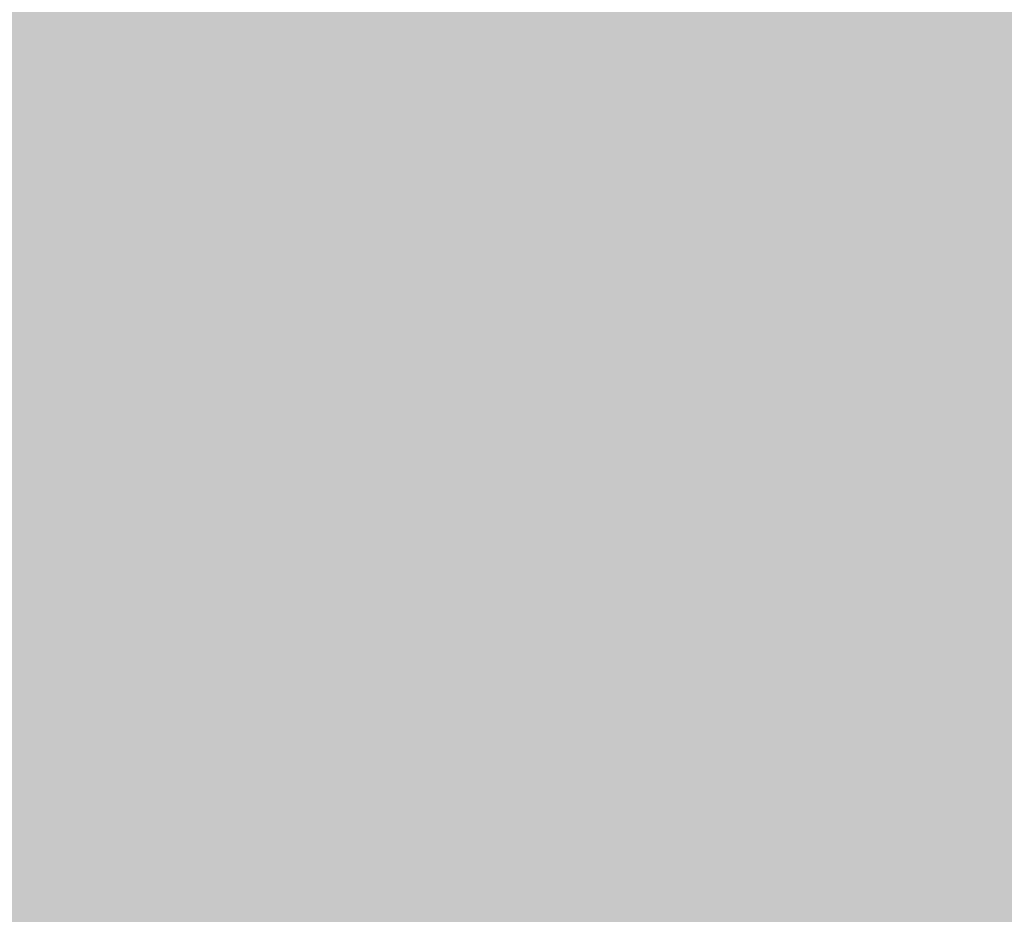
# Model space of a CAD drawing. Units: inches. Extents: x 2083 to 3317, y 1141 to 2115.
# Tile 42 of 256: x 2236.512 to 2237.1059, y 1477.1165 to 1477.6562. Entities that reach past the tile are written whole.
import ezdxf

# ---------------------------------------------------------------- set-up
doc = ezdxf.new("R2010")
doc.units = ezdxf.units.IN
doc.layers.add('A-ANNO-DIMS', color=2, linetype='Continuous', lineweight=18)
doc.layers.add('A-WALL-PATT', color=251, linetype='Continuous', lineweight=13, true_color=0x636466)
doc.styles.get("Standard").update_dxf_attribs({"font": 'arial.ttf'})
doc.dimstyles.new('ISO-25', dxfattribs={"dimtxt": 12, "dimasz": 12, "dimexe": 1.25, "dimexo": 0.625, "dimtad": 1, "dimlunit": 3, "dimtxsty": 'Standard', "dimcen": 2.5, "dimadec": 0, "dimazin": 0, "dimtfac": 1, "dimtmove": 0, "dimatfit": 3, "dimfxl": 1, "dimarcsym": 0})

# ---------------------------------------------------------------- blocks, each defined once
blk = doc.blocks.new('*D30')
at = {"layer": 'A-ANNO-DIMS', "color": 0, "lineweight": -2, "transparency": 16777216}
for p, q in [((2240.01786, 1445.27381), (2240.01786, 1448.04553)), ((2254.32933, 1445.27381), (2254.32933, 1448.04553)), ((2228.01786, 1446.79553), (2216.01786, 1446.79553)), ((2240.01786, 1446.79553), (2254.32933, 1446.79553)), ((2266.32933, 1446.79553), (2413.76487, 1446.79553))]:
    blk.add_line(p, q, dxfattribs=at)
at = {"layer": 'A-ANNO-DIMS', "color": 0, "transparency": 16777216}
for points in [[(2228.01786, 1448.79553), (2228.01786, 1444.79553), (2240.01786, 1446.79553)], [(2266.32933, 1448.79553), (2266.32933, 1444.79553), (2254.32933, 1446.79553)]]:
    blk.add_solid(points, dxfattribs=at)
at = {"layer": 'Defpoints', "color": 0, "transparency": 16777216}
for p in [(2254.32933, 1446.79553), (2240.01786, 1444.64881), (2254.32933, 1444.64881)]:
    blk.add_point(p, dxfattribs=at)
at = {"layer": 'A-ANNO-DIMS', "color": 0, "transparency": 16777216, "insert": (2346.0471, 1453.62517), "char_height": 12, "attachment_point": 5}
blk.add_mtext('WC 1\'-2 1/2" TYP.', dxfattribs=at)
blk = doc.blocks.new('*D31')
at = {"layer": 'A-ANNO-DIMS', "color": 0, "lineweight": -2, "transparency": 16777216}
for p, q in [((2237.87114, 1456.64881), (2237.87114, 1541.91518)), ((2239.39286, 1444.64881), (2236.62114, 1444.64881)), ((2237.87114, 1431.54754), (2237.87114, 1444.64881)), ((2239.39286, 1431.54754), (2236.62114, 1431.54754)), ((2237.87114, 1419.54754), (2237.87114, 1407.54754))]:
    blk.add_line(p, q, dxfattribs=at)
at = {"layer": 'A-ANNO-DIMS', "color": 0, "transparency": 16777216}
for points in [[(2235.87114, 1456.64881), (2239.87114, 1456.64881), (2237.87114, 1444.64881)], [(2235.87114, 1419.54754), (2239.87114, 1419.54754), (2237.87114, 1431.54754)]]:
    blk.add_solid(points, dxfattribs=at)
at = {"layer": 'Defpoints', "color": 0, "transparency": 16777216}
for p in [(2237.87114, 1444.64881), (2240.01786, 1444.64881), (2240.01786, 1431.54754)]:
    blk.add_point(p, dxfattribs=at)
at = {"layer": 'A-ANNO-DIMS', "color": 0, "transparency": 16777216, "insert": (2231.21749, 1505.28199), "char_height": 12, "attachment_point": 5, "rotation": 90}
blk.add_mtext('1\'-1" TYP.', dxfattribs=at)

msp = doc.modelspace()

# ---------------------------------------------------------------- hatches: boundary and pattern name
at = {"layer": 'A-WALL-PATT'}
h = msp.add_hatch(color=256, dxfattribs=at)
h.dxf.hatch_style = 1
h.paths.add_polyline_path([(3126.95978, 2020.76136), (2748.95978, 2020.76136), (2604.95978, 2020.76136), (2226.95978, 2020.76136), (2226.95978, 1702.76136), (2466.95978, 1702.76136), (2466.95978, 1582.76136), (2418.95978, 1582.76136), (2418.95978, 1477.76136), (2226.95978, 1477.76136), (2226.95978, 1263.26136), (2544.95978, 1263.26136), (2544.95978, 1411.76136), (2604.95978, 1411.76136), (2685.95978, 1411.76136), (2685.95978, 1420.76136), (2604.95978, 1420.76136), (2604.95978, 1573.76136), (2604.95978, 1702.76136), (2604.95978, 2011.76136), (2748.95978, 2011.76136), (2748.95978, 1702.76136), (2862.95978, 1702.76136), (2862.95978, 1621.76136), (2871.95978, 1621.76136), (2871.95978, 1702.76136), (2883.95978, 1702.76136), (2883.95978, 1706.93946, -0.026459), (2883.95978, 1711.76136), (2757.95978, 1711.76136), (2757.95978, 1807.76136), (2787.95978, 1807.76136), (2787.95978, 1812.26136), (2757.95978, 1812.26136), (2757.95978, 2011.76136), (2877.95978, 2011.76136), (2877.95978, 1812.26136), (2847.95978, 1812.26136), (2847.95978, 1807.76136), (2889.83574, 1807.76136), (2889.83574, 1812.26136), (2882.45978, 1812.26136), (2882.45978, 2011.76136), (3117.95978, 2011.76136), (3117.95978, 1812.26136), (2937.83574, 1812.26136), (2937.83574, 1807.76136), (2995.70978, 1807.76136), (2995.70978, 1796.11767), (3000.20978, 1796.11767), (3000.20978, 1807.76136), (3117.95978, 1807.76136), (3117.95978, 1711.76136), (3000.20978, 1711.76136), (3000.20978, 1760.11767), (2998.5727, 1760.11767, -0.020711), (2995.70978, 1760.11767), (2995.70978, 1711.76136), (2931.95978, 1711.76136), (2931.95978, 1702.76136), (3126.95978, 1702.76136)])
h.paths.add_polyline_path([(2471.45978, 2011.76136), (2471.45978, 1810.01136), (2462.71694, 1810.01136), (2462.71694, 1805.51136), (2505.95978, 1805.51136), (2505.95978, 1810.01136), (2475.95978, 1810.01136), (2475.95978, 2011.76136), (2595.95978, 2011.76136), (2595.95978, 1810.01136), (2565.95978, 1810.01136), (2565.95978, 1805.51136), (2595.95978, 1805.51136), (2595.95978, 1711.76136), (2235.95978, 1711.76136), (2235.95978, 1805.51136), (2353.70978, 1805.51136), (2353.70978, 1796.05416), (2358.20978, 1796.05416), (2358.20978, 1805.51136), (2414.71694, 1805.51136), (2414.71694, 1810.01136), (2235.95978, 1810.01136), (2235.95978, 2011.76136)], flags=16)
h.paths.add_polyline_path([(2270.20473, 1994.61001), (2270.20473, 1970.61001), (2246.20473, 1970.61001), (2246.20473, 1994.61001)], flags=0)
edge = h.paths.add_edge_path(flags=0)
edge.add_ellipse((2332.02739, 1899.79818), major_axis=(-3.04299, 3.04299), ratio=0.1682525, start_angle=-161.33217, end_angle=-156.30711, ccw=False)
edge.add_ellipse((2333.08204, 1898.74353), major_axis=(-1.05465, 1.05465), ratio=0.4535321, start_angle=-123.37102, end_angle=-94.15911)
edge = h.paths.add_edge_path(flags=0)
edge.add_ellipse((2332.02739, 1968.87629), major_axis=(3.04299, 3.04299), ratio=0.1682525, start_angle=18.66783, end_angle=23.69289)
edge.add_spline(control_points=[(2332.9256, 1970.6911), (2332.22677, 1970.3361), (2330.89371, 1969.65891), (2328.41308, 1970.93214), (2327.20393, 1967.74871), (2324.7096, 1969.95559), (2322.53282, 1967.01235), (2320.01285, 1971.29581), (2317.68031, 1968.15784), (2316.04053, 1967.10205), (2315.4269, 1966.8096)], knot_values=[0, 0, 0, 0, 2.267059, 4.324559, 6.685584, 8.878641, 11.121502, 14.300359, 17.755284, 19.732645, 19.732645, 19.732645, 19.732645], degree=3, periodic=0)
edge.add_ellipse((2332.02739, 1968.87629), major_axis=(3.04299, 3.04299), ratio=0.1682525, start_angle=18.66783, end_angle=23.69289, ccw=False)
edge.add_ellipse((2333.08204, 1969.93094), major_axis=(1.05465, 1.05465), ratio=0.4535321, start_angle=56.62898, end_angle=85.84089, ccw=False)
edge = h.paths.add_edge_path(flags=0)
edge.add_spline(control_points=[(2296.42829, 1967.98791), (2293.6278, 1965.33631), (2287.70362, 1959.72709), (2299.74386, 1949.9957), (2294.53259, 1935.66853), (2290.57323, 1920.60351), (2293.39412, 1909.97369), (2296.18541, 1904.96654)], knot_values=[0.099185, 0.099185, 0.099185, 0.099185, 0.345301, 0.619822, 0.982653, 1.386093, 1.810555, 1.810555, 1.810555, 1.810555], degree=3, periodic=0)
edge.add_spline(control_points=[(2296.18541, 1904.96654), (2297.38358, 1902.6193), (2298.00097, 1901.94931), (2298.55297, 1901.46815)], knot_values=[0.006246, 0.006246, 0.006246, 0.006246, 0.055476, 0.055476, 0.055476, 0.055476], degree=3, periodic=0)
edge.add_spline(control_points=[(2298.55297, 1901.46815), (2297.25861, 1900.92322), (2295.22529, 1900.23213), (2293.06023, 1900.61421), (2292.10142, 1900.78841), (2292.08958, 1900.79057)], knot_values=[0.312835, 0.312835, 0.312835, 0.312835, 0.40178, 0.474987, 0.475903, 0.475903, 0.475903, 0.475903], degree=3, periodic=0)
edge.add_arc((2292.79365, 1904.66411), 3.93701, 215.4209, 259.69818, ccw=False)
edge.add_spline(control_points=[(2289.58531, 1902.3823), (2289.47665, 1902.53509), (2289.36848, 1902.68804), (2289.26086, 1902.84117)], knot_values=[0.102872, 0.102872, 0.102872, 0.102872, 0.116896, 0.116896, 0.116896, 0.116896], degree=3, periodic=0)
edge.add_spline(control_points=[(2289.26086, 1902.84117), (2288.6866, 1902.55019), (2287.64005, 1902.0199), (2285.88134, 1901.87395), (2283.85297, 1901.50435), (2281.71999, 1899.71054), (2278.46699, 1899.49294), (2276.15714, 1901.8832), (2272.25895, 1899.80407), (2267.77761, 1901.84318), (2262.24388, 1900.18403), (2257.41493, 1901.78206), (2254.31837, 1900.72612), (2253.17828, 1900.33734)], knot_values=[0, 0, 0, 0, 1.907977, 3.477176, 5.261074, 7.972851, 11.680248, 13.717921, 16.939592, 22.789562, 27.502503, 33.595215, 37.145618, 37.145618, 37.145618, 37.145618], degree=3, periodic=0)
edge.add_line((2253.17828, 1900.33734), (2250.24424, 1902.84117))
edge.add_line((2250.24424, 1902.84117), (2250.24424, 1965.8333))
edge.add_line((2250.24424, 1965.8333), (2253.17828, 1968.33712))
edge.add_spline(control_points=[(2253.17828, 1968.33712), (2254.31837, 1967.94835), (2257.41493, 1966.89241), (2262.24388, 1968.49043), (2267.77761, 1966.83128), (2271.52673, 1968.53722), (2273.87591, 1967.82829), (2274.2067, 1967.72764)], knot_values=[0, 0, 0, 0, 0.09018, 0.244935, 0.364644, 0.513233, 0.537855, 0.537855, 0.537855, 0.537855], degree=3, periodic=0)
edge.add_arc((2274.35289, 1963.79335), 3.93701, 72.05113, 92.12795, ccw=False)
edge.add_arc((2281.29693, 1985.23), 18.5963, 252.051134, 288.565722)
edge.add_arc((2292.31672, 1956.02888), 12.64608, 71.026788, 113.778218, ccw=False)
edge = h.paths.add_edge_path(flags=0)
edge.add_spline(control_points=[(2274.89941, 1951.85619), (2275.06616, 1951.61659), (2275.23269, 1951.37659), (2275.39799, 1951.13585)], knot_values=[1.409916, 1.409916, 1.409916, 1.409916, 1.43159, 1.43159, 1.43159, 1.43159], degree=3, periodic=0)
edge.add_spline(control_points=[(2275.39799, 1951.13585), (2275.79211, 1950.56189), (2276.17923, 1949.98377), (2276.54555, 1949.3971)], knot_values=[1.358238, 1.358238, 1.358238, 1.358238, 1.409916, 1.409916, 1.409916, 1.409916], degree=3, periodic=0)
edge.add_line((2276.54555, 1949.3971), (2277.43729, 1947.86218))
edge.add_spline(control_points=[(2277.43729, 1947.86218), (2276.30383, 1945.67311), (2274.6397, 1942.42688), (2274.63161, 1938.0939), (2272.79912, 1930.85155), (2274.35643, 1943.89705), (2275.94768, 1947.92336), (2276.54555, 1949.3971)], knot_values=[0.005632, 0.005632, 0.005632, 0.005632, 0.186014, 0.266002, 0.357087, 0.59639, 0.739732, 0.739732, 0.739732, 0.739732], degree=3, periodic=0)
edge.add_spline(control_points=[(2276.54555, 1949.3971), (2276.17923, 1949.98377), (2275.79211, 1950.56189), (2275.39799, 1951.13585)], knot_values=[1.358238, 1.358238, 1.358238, 1.358238, 1.409916, 1.409916, 1.409916, 1.409916], degree=3, periodic=0)
edge.add_spline(control_points=[(2275.39799, 1951.13585), (2274.9425, 1950.08045), (2274.20776, 1948.02527), (2273.9346, 1944.85148), (2272.46853, 1937.62749), (2273.46622, 1945.69647), (2274.70062, 1951.05947), (2274.89941, 1951.85619)], knot_values=[0.104364, 0.104364, 0.104364, 0.104364, 0.189636, 0.269624, 0.36071, 0.600013, 0.644622, 0.644622, 0.644622, 0.644622], degree=3, periodic=0)
h.paths.add_polyline_path([(2269.16751, 1963.12757, -0.357527), (2268.17063, 1960.97637, -0.092561), (2268.17063, 1939.43632, -0.357527), (2269.16751, 1937.28512, -0.357527), (2267.01631, 1938.282, -0.164785), (2254.68558, 1938.282, -0.357527), (2252.53438, 1937.28512, -0.357527), (2253.53126, 1939.43632, -0.092561), (2253.53126, 1960.97637, -0.357527), (2252.53438, 1963.12757, -0.357527), (2254.68558, 1962.13069, -0.164785), (2267.01631, 1962.13069, -0.357527)], flags=0)
h.paths.add_polyline_path([(2248.87407, 1967.8018), (2248.87407, 1957.02771), (2249.45778, 1957.02771), (2249.45778, 1911.64676), (2248.87407, 1911.64676), (2248.87407, 1900.87267), (2246.51186, 1900.87267, 0.197327), (2244.14966, 1902.45687), (2244.14966, 1966.21759, 0.197327), (2246.51186, 1967.8018)], flags=0)
h.paths.add_polyline_path([(2269.16751, 1931.38934, -0.357527), (2268.17063, 1929.23814, -0.092561), (2268.17063, 1907.6981, -0.357527), (2269.16751, 1905.54689, -0.357527), (2267.01631, 1906.54377, -0.164785), (2254.68558, 1906.54377, -0.357527), (2252.53438, 1905.54689, -0.357527), (2253.53126, 1907.6981, -0.092561), (2253.53126, 1929.23814, -0.357527), (2252.53438, 1931.38934, -0.357527), (2254.68558, 1930.39246, -0.164785), (2267.01631, 1930.39246, -0.357527)], flags=0)
edge = h.paths.add_edge_path(flags=0)
edge.add_spline(control_points=[(2276.19686, 1906.7237), (2276.16814, 1909.02893), (2276.11405, 1913.37185), (2270.59842, 1924.92498), (2273.90517, 1919.01278), (2275.92171, 1916.26206), (2275.47457, 1912.40215), (2277.25787, 1910.38062), (2276.69604, 1908.22504), (2276.64622, 1906.81302), (2276.61782, 1906.00841)], knot_values=[0, 0, 0, 0, 8.61026, 16.221274, 18.843057, 23.804898, 27.440828, 29.356102, 31.203478, 33.650687, 33.650687, 33.650687, 33.650687], degree=3, periodic=0)
edge.add_spline(control_points=[(2276.61782, 1906.00841), (2276.62331, 1905.62414), (2276.49774, 1904.62866), (2275.44178, 1903.85473), (2274.93731, 1903.08045), (2274.85908, 1902.84117)], knot_values=[0.156488, 0.156488, 0.156488, 0.156488, 0.184398, 0.231376, 0.250598, 0.250598, 0.250598, 0.250598], degree=3, periodic=0)
edge.add_line((2274.85908, 1902.84117), (2276.50598, 1902.84117))
edge.add_spline(control_points=[(2276.50598, 1902.84117), (2276.78831, 1903.08494), (2277.66507, 1904.1252), (2278.24954, 1904.34074), (2277.65387, 1908.52739), (2278.15567, 1906.22781), (2278.10046, 1905.28595), (2278.84667, 1904.06901), (2277.85679, 1903.41495), (2277.87419, 1902.99105), (2277.90356, 1902.84117)], knot_values=[0.059574, 0.059574, 0.059574, 0.059574, 0.080753, 0.103741, 0.16972, 0.176036, 0.207137, 0.240474, 0.262341, 0.27366, 0.27366, 0.27366, 0.27366], degree=3, periodic=0)
edge.add_line((2277.90356, 1902.84117), (2280.02983, 1902.84117))
edge.add_spline(control_points=[(2280.02983, 1902.84117), (2279.88822, 1903.0884), (2279.49926, 1903.98155), (2280.15228, 1905.93935), (2278.10362, 1909.65776), (2279.76239, 1907.18529), (2280.3279, 1904.87486), (2280.48511, 1903.48959), (2281.46327, 1903.24943), (2281.75834, 1902.9365), (2281.83404, 1902.84117)], knot_values=[0.013856, 0.013856, 0.013856, 0.013856, 0.034874, 0.088867, 0.107879, 0.126738, 0.158714, 0.193757, 0.217487, 0.226722, 0.226722, 0.226722, 0.226722], degree=3, periodic=0)
edge.add_spline(control_points=[(2281.83404, 1902.84117), (2281.78753, 1902.8267), (2281.64702, 1902.78299), (2281.39553, 1902.85949), (2281.08808, 1902.98524), (2280.72068, 1903.0609), (2280.33345, 1903.02573), (2280.12477, 1902.89888), (2280.02983, 1902.84117)], knot_values=[0, 0, 0, 0, 0.14413, 0.435517, 0.749276, 1.153046, 1.548371, 1.878348, 1.878348, 1.878348, 1.878348], degree=3, periodic=0)
edge.add_line((2280.02983, 1902.84117), (2277.90356, 1902.84117))
edge.add_spline(control_points=[(2277.90356, 1902.84117), (2277.89286, 1902.79586), (2277.8654, 1902.67964), (2277.60748, 1902.68748), (2277.27405, 1902.8007), (2276.83792, 1902.61977), (2276.58381, 1902.78926), (2276.50598, 1902.84117)], knot_values=[0, 0, 0, 0, 0.127189, 0.326199, 0.628009, 1.24357, 1.515331, 1.515331, 1.515331, 1.515331], degree=3, periodic=0)
edge.add_line((2276.50598, 1902.84117), (2274.85908, 1902.84117))
edge.add_spline(control_points=[(2274.85908, 1902.84117), (2274.81444, 1902.89859), (2274.72513, 1903.01345), (2274.49348, 1903.11897), (2274.24429, 1902.96054), (2273.93712, 1903.18494), (2273.61404, 1902.98314), (2273.40832, 1902.88304), (2273.32225, 1902.84117)], knot_values=[0, 0, 0, 0, 0.21843, 0.436957, 0.687977, 0.990379, 1.398396, 1.69185, 1.69185, 1.69185, 1.69185], degree=3, periodic=0)
edge.add_spline(control_points=[(2273.32225, 1902.84117), (2273.61674, 1903.44569), (2274.274, 1904.53825), (2276.02724, 1904.5737), (2276.20696, 1906.58364), (2276.19686, 1906.7237)], knot_values=[0.012227, 0.012227, 0.012227, 0.012227, 0.059472, 0.106218, 0.134458, 0.134458, 0.134458, 0.134458], degree=3, periodic=0)
h.paths.add_polyline_path([(2270.77605, 1897.78983), (2270.77605, 1873.78983), (2246.77605, 1873.78983), (2246.77605, 1897.78983)], flags=0)
h.paths.add_polyline_path([(2353.70978, 1760.00506), (2353.70978, 1760.05416), (2358.20978, 1760.05416, -0.033729)], flags=0)
h.paths.add_polyline_path([(2321.81912, 1737.52919), (2341.99533, 1737.52919, -0.414214), (2343.20327, 1736.32124), (2343.20327, 1721.0206, -0.414214), (2341.99533, 1719.81265), (2321.81912, 1719.81265, -0.414214), (2320.61117, 1721.0206), (2320.61117, 1736.32124, -0.414214)], flags=0)
h.paths.add_polyline_path([(2324.23501, 1736.32124), (2339.57944, 1736.32124, -0.414214), (2341.99533, 1733.90535), (2341.99533, 1725.44973, -0.414214), (2339.57944, 1723.03384), (2333.68059, 1723.03384), (2333.84532, 1722.04547, -0.870646), (2335.4254, 1721.82589, -0.767327), (2333.92269, 1721.42324), (2331.29102, 1721.42324, -0.767327), (2329.78832, 1721.82589, -0.870646), (2331.3684, 1722.04547), (2331.53313, 1723.03384), (2324.23501, 1723.03384, -0.414214), (2321.81912, 1725.44973), (2321.81912, 1733.90535, -0.414214)], flags=0)
h.paths.add_polyline_path([(2570.48379, 1928.61544), (2589.68379, 1928.61544), (2590.16883, 1928.61544), (2590.16883, 1904.9934), (2570.48379, 1904.9934)], flags=0)
h.paths.add_polyline_path([(2574.44732, 1927.26382, -1), (2572.82884, 1927.26382, -1)], flags=0)
h.paths.add_polyline_path([(2573.08987, 1926.94088), (2573.92503, 1927.77604), (2574.14774, 1927.55333), (2573.31258, 1926.71817)], flags=0)
h.paths.add_polyline_path([(2578.77906, 1919.72962, -1), (2571.59166, 1919.72962, -1)], flags=0)
h.paths.add_polyline_path([(2578.38536, 1919.72962, -1), (2571.98536, 1919.72962, -1)], flags=0)
h.paths.add_polyline_path([(2331.59576, 1729.47622, -1), (2333.61795, 1729.47622, -1)], flags=0)
h.paths.add_polyline_path([(2578.03423, 1927.26382, -1), (2576.41574, 1927.26382, -1)], flags=0)
h.paths.add_polyline_path([(2576.68885, 1927.53109), (2576.91156, 1927.7538), (2577.74673, 1926.91863), (2577.52402, 1926.69592)], flags=0)
h.paths.add_polyline_path([(2578.13906, 1909.85954, -1), (2572.23166, 1909.85954, -1)], flags=0)
h.paths.add_polyline_path([(2577.74536, 1909.85954, -1), (2572.62536, 1909.85954, -1)], flags=0)
h.paths.add_polyline_path([(2583.79772, 1927.26382, -1), (2582.17923, 1927.26382, -1)], flags=0)
h.paths.add_polyline_path([(2582.71865, 1927.7538), (2583.55381, 1926.91863), (2583.3311, 1926.69592), (2582.49594, 1927.53109)], flags=0)
h.paths.add_polyline_path([(2582.49594, 1927.53109), (2582.71865, 1927.7538), (2583.55381, 1926.91863), (2583.3311, 1926.69592)], flags=0)
h.paths.add_polyline_path([(2587.73906, 1920.52962, -1), (2581.83166, 1920.52962, -1)], flags=0)
h.paths.add_polyline_path([(2587.34536, 1920.52962, -1), (2582.22536, 1920.52962, -1)], flags=0)
h.paths.add_polyline_path([(2587.38462, 1927.26382, -1), (2585.76613, 1927.26382, -1)], flags=0)
h.paths.add_polyline_path([(2586.08199, 1926.98025), (2586.91716, 1927.81541), (2587.13987, 1927.5927), (2586.3047, 1926.75754)], flags=0)
h.paths.add_polyline_path([(2588.37906, 1910.65954, -1), (2581.19166, 1910.65954, -1)], flags=0)
h.paths.add_polyline_path([(2587.98536, 1910.65954, -1), (2581.58536, 1910.65954, -1)], flags=0)
h.paths.add_polyline_path([(2417.16773, 1729.4779), (2437.34394, 1729.4779, -0.414214), (2438.55188, 1728.26995), (2438.55188, 1712.96931, -0.414214), (2437.34394, 1711.76136), (2417.16773, 1711.76136, -0.414214), (2415.95978, 1712.96931), (2415.95978, 1728.26995, -0.414214)], flags=0)
h.paths.add_polyline_path([(2419.58362, 1728.26995), (2434.92805, 1728.26995, -0.414214), (2437.34394, 1725.85406), (2437.34394, 1717.39844, -0.414214), (2434.92805, 1714.98255), (2429.0292, 1714.98255), (2429.19393, 1713.99418, -0.870646), (2430.77401, 1713.7746, -0.767327), (2429.2713, 1713.37195), (2426.63963, 1713.37195, -0.767327), (2425.13693, 1713.7746, -0.870646), (2426.71701, 1713.99418), (2426.88174, 1714.98255), (2419.58362, 1714.98255, -0.414214), (2417.16773, 1717.39844), (2417.16773, 1725.85406, -0.414214)], flags=0)
h.paths.add_polyline_path([(2419.58362, 1728.26995), (2434.92805, 1728.26995, -0.414214), (2437.34394, 1725.85406), (2437.34394, 1717.39844, -0.414214), (2434.92805, 1714.98255), (2429.0292, 1714.98255), (2428.35812, 1719.00903), (2427.55282, 1719.00903), (2426.88174, 1714.98255), (2419.58362, 1714.98255, -0.414214), (2417.16773, 1717.39844), (2417.16773, 1725.85406, -0.414214)], flags=0)
h.paths.add_polyline_path([(2426.94437, 1721.42492, -1), (2428.96656, 1721.42492, -1)], flags=0)
h.paths.add_polyline_path([(2475.95978, 1702.76136), (2595.95978, 1702.76136), (2595.95978, 1582.76136), (2475.95978, 1582.76136)], flags=16)
h.paths.add_polyline_path([(2427.95978, 1573.76136), (2595.95978, 1573.76136), (2595.95978, 1468.76136), (2595.95978, 1420.76136), (2384.45978, 1420.76136), (2384.45978, 1468.76136), (2427.95978, 1468.76136)], flags=16)
h.paths.add_polyline_path([(2379.95978, 1468.76136), (2379.95978, 1420.76136), (2235.95978, 1420.76136), (2235.95978, 1468.76136)], flags=16)
h.paths.add_polyline_path([(2317.816, 1466.69577), (2337.9922, 1466.69577, -0.414214), (2339.20015, 1465.48782), (2339.20015, 1450.18718, -0.414214), (2337.9922, 1448.97923), (2317.816, 1448.97923, -0.414214), (2316.60805, 1450.18718), (2316.60805, 1465.48782, -0.414214)], flags=0)
h.paths.add_polyline_path([(2320.23189, 1465.48782), (2335.57631, 1465.48782, -0.414214), (2337.9922, 1463.07193), (2337.9922, 1454.61631, -0.414214), (2335.57631, 1452.20042), (2329.67747, 1452.20042), (2329.84219, 1451.21205, -0.870646), (2331.42228, 1450.99247, -0.767327), (2329.91957, 1450.58983), (2327.2879, 1450.58983, -0.767327), (2325.7852, 1450.99247, -0.870646), (2327.36528, 1451.21205), (2327.53001, 1452.20042), (2320.23189, 1452.20042, -0.414214), (2317.816, 1454.61631), (2317.816, 1463.07193, -0.414214)], flags=0)
h.paths.add_polyline_path([(2320.23189, 1465.48782), (2335.57631, 1465.48782, -0.414214), (2337.9922, 1463.07193), (2337.9922, 1454.61631, -0.414214), (2335.57631, 1452.20042), (2329.67747, 1452.20042), (2329.00638, 1456.22691), (2328.20109, 1456.22691), (2327.53001, 1452.20042), (2320.23189, 1452.20042, -0.414214), (2317.816, 1454.61631), (2317.816, 1463.07193, -0.414214)], flags=0)
h.paths.add_polyline_path([(2327.59264, 1458.6428, -1), (2329.61483, 1458.6428, -1)], flags=0)
h.paths.add_polyline_path([(2244.41174, 1433.34045), (2241.92094, 1433.34045, -0.414214), (2240.01786, 1435.24354), (2240.01786, 1440.95281, -0.414211), (2241.92093, 1442.8559), (2244.41174, 1442.8559, -1.976472)], flags=0)
h.paths.add_polyline_path([(2245.35689, 1434.39754, -0.414214), (2245.35689, 1441.79881, -2.144098)], flags=0)
h.paths.add_polyline_path([(2535.95978, 1416.26136), (2535.95978, 1272.26136), (2235.95978, 1272.26136), (2235.95978, 1416.26136)], flags=16)
h.paths.add_polyline_path([(2260.11956, 1384.29284), (2260.11956, 1362.03865), (2237.86537, 1362.03865), (2237.86537, 1384.29284)], flags=0)
edge = h.paths.add_edge_path(flags=0)
edge.add_line((2318.25185, 1362.0933), (2318.1458, 1362.00097))
edge.add_ellipse((2317.44512, 1360.43104), major_axis=(2.82164, 2.82164), ratio=0.1682525, start_angle=18.66783, end_angle=20.94813, ccw=False)
edge.add_ellipse((2318.42305, 1361.40897), major_axis=(0.97793, 0.97793), ratio=0.4535321, start_angle=56.62898, end_angle=70.2262, ccw=False)
edge = h.paths.add_edge_path(flags=0)
edge.add_line((2319.10737, 1295.57108), (2319.01504, 1295.67713))
edge.add_ellipse((2317.44512, 1296.37781), major_axis=(-2.82164, 2.82164), ratio=0.1682525, start_angle=-161.33217, end_angle=-159.05187, ccw=False)
edge.add_ellipse((2318.42305, 1295.39988), major_axis=(-0.97793, 0.97793), ratio=0.4535321, start_angle=-123.37102, end_angle=-109.7738)
edge = h.paths.add_edge_path(flags=0)
edge.add_spline(control_points=[(2284.21035, 1301.17022), (2284.58069, 1300.44472), (2284.89119, 1299.89202), (2285.15955, 1299.46102)], knot_values=[0.039066, 0.039066, 0.039066, 0.039066, 0.055476, 0.055476, 0.055476, 0.055476], degree=3, periodic=0)
edge.add_line((2285.15955, 1299.46102), (2284.21035, 1301.17022))
edge = h.paths.add_edge_path(flags=0)
edge.add_line((2280.41246, 1297.29801), (2283.36999, 1297.03612))
edge.add_line((2283.36999, 1297.03612), (2286.40569, 1297.92631))
edge.add_spline(control_points=[(2286.40569, 1297.92631), (2285.30549, 1297.46312), (2284.34478, 1297.12915), (2283.36999, 1297.03612)], knot_values=[0.394369, 0.394369, 0.394369, 0.394369, 0.475903, 0.475903, 0.475903, 0.475903], degree=3, periodic=0)
edge.add_spline(control_points=[(2283.36999, 1297.03612), (2283.28139, 1297.02767), (2282.31629, 1296.95734), (2281.3125, 1297.13448), (2280.42344, 1297.29602), (2280.41246, 1297.29801)], knot_values=[0.312835, 0.312835, 0.312835, 0.312835, 0.320246, 0.393453, 0.394369, 0.394369, 0.394369, 0.394369], degree=3, periodic=0)
edge = h.paths.add_edge_path(flags=0)
edge.add_line((2284.43556, 1359.60729), (2280.44629, 1355.32805))
edge.add_line((2280.44629, 1355.32805), (2279.57999, 1351.01775))
edge.add_line((2279.57999, 1351.01775), (2282.41297, 1346.58043))
edge.add_spline(control_points=[(2282.41297, 1346.58043), (2283.15333, 1345.58924), (2284.2529, 1344.0289), (2284.80104, 1342.38717), (2284.93516, 1341.80554)], knot_values=[1.240098, 1.240098, 1.240098, 1.240098, 1.332892, 1.382712, 1.382712, 1.382712, 1.382712], degree=3, periodic=0)
edge.add_spline(control_points=[(2284.93516, 1341.80554), (2285.31911, 1340.1406), (2285.23303, 1338.4092), (2284.90994, 1336.65412)], knot_values=[1.097484, 1.097484, 1.097484, 1.097484, 1.240098, 1.240098, 1.240098, 1.240098], degree=3, periodic=0)
edge.add_spline(control_points=[(2284.90994, 1336.65412), (2284.58685, 1334.89904), (2284.02675, 1333.12027), (2283.46264, 1331.36058)], knot_values=[0.95487, 0.95487, 0.95487, 0.95487, 1.097484, 1.097484, 1.097484, 1.097484], degree=3, periodic=0)
edge.add_line((2283.46264, 1331.36058), (2281.89038, 1326.15336))
edge.add_line((2281.89038, 1326.15336), (2280.75626, 1321.05609))
edge.add_line((2280.75626, 1321.05609), (2280.2992, 1316.00198))
edge.add_line((2280.2992, 1316.00198), (2280.71593, 1310.95007))
edge.add_line((2280.71593, 1310.95007), (2282.02809, 1305.97214))
edge.add_line((2282.02809, 1305.97214), (2284.21035, 1301.17022))
edge.add_spline(control_points=[(2284.21035, 1301.17022), (2283.34073, 1302.73019), (2282.6119, 1304.33649), (2282.02809, 1305.97214)], knot_values=[0.099185, 0.099185, 0.099185, 0.099185, 0.241799, 0.241799, 0.241799, 0.241799], degree=3, periodic=0)
edge.add_spline(control_points=[(2282.02809, 1305.97214), (2281.44428, 1307.60778), (2281.00549, 1309.27276), (2280.71593, 1310.95007)], knot_values=[0.241799, 0.241799, 0.241799, 0.241799, 0.384413, 0.384413, 0.384413, 0.384413], degree=3, periodic=0)
edge.add_spline(control_points=[(2280.71593, 1310.95007), (2280.43324, 1312.58761), (2280.28939, 1314.27696), (2280.29889, 1315.96203), (2280.2992, 1316.00198)], knot_values=[0.384413, 0.384413, 0.384413, 0.384413, 0.523647, 0.527028, 0.527028, 0.527028, 0.527028], degree=3, periodic=0)
edge.add_spline(control_points=[(2280.2992, 1316.00198), (2280.31233, 1317.68696), (2280.47787, 1319.36793), (2280.75626, 1321.05609)], knot_values=[0.527028, 0.527028, 0.527028, 0.527028, 0.669642, 0.669642, 0.669642, 0.669642], degree=3, periodic=0)
edge.add_spline(control_points=[(2280.75626, 1321.05609), (2281.03465, 1322.74425), (2281.42588, 1324.43961), (2281.89038, 1326.15336)], knot_values=[0.669642, 0.669642, 0.669642, 0.669642, 0.812256, 0.812256, 0.812256, 0.812256], degree=3, periodic=0)
edge.add_spline(control_points=[(2281.89038, 1326.15336), (2282.26438, 1327.53325), (2282.78787, 1329.26181), (2283.35275, 1331.01778), (2283.46264, 1331.36058)], knot_values=[0.812256, 0.812256, 0.812256, 0.812256, 0.927087, 0.95487, 0.95487, 0.95487, 0.95487], degree=3, periodic=0)
edge.add_line((2283.46264, 1331.36058), (2284.90994, 1336.65412))
edge.add_line((2284.90994, 1336.65412), (2284.93516, 1341.80554))
edge.add_line((2284.93516, 1341.80554), (2282.41297, 1346.58043))
edge.add_spline(control_points=[(2282.41297, 1346.58043), (2281.27513, 1348.10379), (2280.07845, 1349.57032), (2279.57999, 1351.01775)], knot_values=[1.382712, 1.382712, 1.382712, 1.382712, 1.525326, 1.525326, 1.525326, 1.525326], degree=3, periodic=0)
edge.add_spline(control_points=[(2279.57999, 1351.01775), (2279.44328, 1351.41472), (2279.13631, 1352.85692), (2279.73519, 1354.29039), (2280.44629, 1355.32805)], knot_values=[1.525326, 1.525326, 1.525326, 1.525326, 1.564439, 1.667941, 1.667941, 1.667941, 1.667941], degree=3, periodic=0)
edge.add_spline(control_points=[(2280.44629, 1355.32805), (2281.42611, 1356.75784), (2282.93084, 1358.18256), (2284.43556, 1359.60729)], knot_values=[1.667941, 1.667941, 1.667941, 1.667941, 1.810555, 1.810555, 1.810555, 1.810555], degree=3, periodic=0)
edge.add_arc((2280.62307, 1348.51818), 11.72618, 71.026788, 113.778218)
edge.add_arc((2270.40489, 1375.59516), 17.24357, 252.051134, 288.565722, ccw=False)
edge.add_arc((2263.96597, 1355.71785), 3.65062, 72.05113, 92.12795)
edge.add_arc((2263.96597, 1355.71785), 3.65062, 92.12795, 177.98513)
edge.add_spline(control_points=[(2260.3176, 1355.8462), (2260.26042, 1354.22067), (2260.55128, 1350.18655), (2262.99934, 1346.76625), (2264.47274, 1344.64902)], knot_values=[1.43159, 1.43159, 1.43159, 1.43159, 1.564144, 1.770695, 1.770695, 1.770695, 1.770695], degree=3, periodic=0)
edge.add_line((2264.47274, 1344.64902), (2264.93559, 1343.98253))
edge.add_spline(control_points=[(2263.80104, 1340.24811), (2263.84324, 1340.51409), (2264.06724, 1341.75647), (2264.51269, 1343.00245), (2264.93505, 1343.98108)], knot_values=[0.53657, 0.53657, 0.53657, 0.53657, 0.559349, 0.644622, 0.644622, 0.644622, 0.644622], degree=3, periodic=0)
edge.add_spline(control_points=[(2264.93505, 1343.98108), (2265.11777, 1343.71497), (2265.29888, 1343.44791), (2265.47676, 1343.17936)], knot_values=[1.384077, 1.384077, 1.384077, 1.384077, 1.409916, 1.409916, 1.409916, 1.409916], degree=3, periodic=0)
edge.add_spline(control_points=[(2265.47676, 1343.17936), (2265.65464, 1342.91082), (2265.8293, 1342.64081), (2265.99913, 1342.36881)], knot_values=[1.358238, 1.358238, 1.358238, 1.358238, 1.384077, 1.384077, 1.384077, 1.384077], degree=3, periodic=0)
edge.add_line((2265.99913, 1342.36881), (2266.82601, 1340.94555))
edge.add_spline(control_points=[(2266.82601, 1340.94555), (2268.8944, 1337.08969), (2271.39817, 1325.843), (2270.51616, 1310.56856), (2275.91938, 1301.86061), (2277.78951, 1299.19945)], knot_values=[0.116896, 0.116896, 0.116896, 0.116896, 0.472987, 1.050969, 1.313793, 1.313793, 1.313793, 1.313793], degree=3, periodic=0)
edge.add_spline(control_points=[(2277.78951, 1299.19945), (2277.83941, 1299.12845), (2277.88943, 1299.0575), (2277.93957, 1298.98658)], knot_values=[0.109884, 0.109884, 0.109884, 0.109884, 0.116896, 0.116896, 0.116896, 0.116896], degree=3, periodic=0)
edge.add_line((2277.93957, 1298.98658), (2277.78885, 1299.19911))
edge.add_spline(control_points=[(2277.78885, 1299.19911), (2277.25658, 1298.92941), (2276.28635, 1298.4379), (2275.03935, 1298.33442), (2274.38333, 1298.2389), (2274.21525, 1298.20934)], knot_values=[33.12187, 33.12187, 33.12187, 33.12187, 35.029056, 36.598255, 37.144827, 37.144827, 37.144827, 37.144827], degree=3, periodic=0)
edge.add_line((2274.21525, 1298.20934), (2273.07315, 1297.89296))
edge.add_spline(control_points=[(2273.07315, 1297.89296), (2272.32294, 1297.57978), (2271.03915, 1296.51051), (2269.24839, 1296.22606), (2268.4231, 1296.37465)], knot_values=[26.532584, 26.532584, 26.532584, 26.532584, 29.198919, 31.839101, 31.839101, 31.839101, 31.839101], degree=3, periodic=0)
edge.add_line((2268.4231, 1296.37465), (2263.8785, 1297.45753))
edge.add_spline(control_points=[(2263.8785, 1297.45753), (2263.55608, 1297.35943), (2261.86031, 1296.83869), (2260.23878, 1297.28241), (2258.93345, 1297.51646)], knot_values=[15.919551, 15.919551, 15.919551, 15.919551, 16.939592, 21.226067, 21.226067, 21.226067, 21.226067], degree=3, periodic=0)
edge.add_line((2258.93345, 1297.51646), (2254.05523, 1297.32901))
edge.add_spline(control_points=[(2254.05523, 1297.32901), (2253.75553, 1297.29582), (2252.11368, 1297.16517), (2250.46187, 1297.54422), (2249.12969, 1297.66788)], knot_values=[5.306517, 5.306517, 5.306517, 5.306517, 6.276435, 10.613034, 10.613034, 10.613034, 10.613034], degree=3, periodic=0)
edge.add_line((2249.12969, 1297.66788), (2244.33165, 1296.87776))
edge.add_line((2244.33165, 1296.87776), (2241.61103, 1299.19945))
edge.add_line((2241.61103, 1299.19945), (2241.61103, 1357.6094))
edge.add_line((2241.61103, 1357.6094), (2244.33165, 1359.9311))
edge.add_line((2244.33165, 1359.9311), (2252.72882, 1359.54269))
edge.add_spline(control_points=[(2252.72882, 1359.54269), (2252.87094, 1359.54644), (2253.30574, 1359.54817), (2253.73984, 1359.51427), (2254.03174, 1359.48243)], knot_values=[0.233291, 0.233291, 0.233291, 0.233291, 0.244935, 0.268927, 0.268927, 0.268927, 0.268927], degree=3, periodic=0)
edge.add_line((2254.03174, 1359.48243), (2259.58719, 1359.41639))
edge.add_spline(control_points=[(2259.58719, 1359.41639), (2260.67707, 1359.6285), (2262.0732, 1359.897), (2263.52369, 1359.45928), (2263.83042, 1359.36595)], knot_values=[0.422516, 0.422516, 0.422516, 0.422516, 0.513233, 0.537855, 0.537855, 0.537855, 0.537855], degree=3, periodic=0)
edge.add_arc((2263.96597, 1355.71785), 3.65062, 72.05113, 92.12795, ccw=False)
edge.add_arc((2270.40489, 1375.59516), 17.24357, 252.051134, 288.565722)
edge.add_arc((2280.62307, 1348.51818), 11.72618, 71.026788, 113.778218, ccw=False)
h.paths.add_polyline_path([(2240.34053, 1359.43471), (2240.34053, 1349.44435), (2240.88178, 1349.44435), (2240.88178, 1307.3645), (2240.34053, 1307.3645), (2240.34053, 1297.37414), (2238.15016, 1297.37414, 0.197327), (2235.95978, 1298.84311), (2235.95978, 1357.96575, 0.197327), (2238.15016, 1359.43471)], flags=0)
h.paths.add_polyline_path([(2259.15779, 1355.1005, -0.357527), (2258.23342, 1353.10578, -0.092561), (2258.23342, 1333.1326, -0.357527), (2259.15779, 1331.13788, -0.357527), (2257.16307, 1332.06225, -0.164785), (2245.7293, 1332.06225, -0.357527), (2243.73458, 1331.13788, -0.357527), (2244.65895, 1333.1326, -0.092561), (2244.65895, 1353.10578, -0.357527), (2243.73458, 1355.1005, -0.357527), (2245.7293, 1354.17613, -0.164785), (2257.16307, 1354.17613, -0.357527)], flags=0)
edge = h.paths.add_edge_path(flags=0)
edge.add_line((2265.99913, 1342.36881), (2266.82601, 1340.94555))
edge.add_line((2266.82601, 1340.94555), (2265.30756, 1337.81407))
edge.add_line((2265.30756, 1337.81407), (2264.35823, 1334.65294))
edge.add_line((2264.35823, 1334.65294), (2264.26201, 1333.7997))
edge.add_spline(control_points=[(2264.26201, 1333.7997), (2264.20836, 1333.18705), (2264.16206, 1332.36553), (2264.00714, 1331.41393), (2263.96905, 1331.20183)], knot_values=[0.464444, 0.464444, 0.464444, 0.464444, 0.516691, 0.531608, 0.531608, 0.531608, 0.531608], degree=3, periodic=0)
edge.add_spline(control_points=[(2263.96905, 1331.20183), (2263.77453, 1330.11887), (2263.42437, 1328.79084), (2263.25742, 1328.53065), (2263.23403, 1328.51461)], knot_values=[0.372682, 0.372682, 0.372682, 0.372682, 0.44885, 0.464444, 0.464444, 0.464444, 0.464444], degree=3, periodic=0)
edge.add_spline(control_points=[(2263.23403, 1328.51461), (2263.09638, 1328.42023), (2263.13117, 1329.30148), (2263.27495, 1330.61575)], knot_values=[0.280919, 0.280919, 0.280919, 0.280919, 0.372682, 0.372682, 0.372682, 0.372682], degree=3, periodic=0)
edge.add_spline(control_points=[(2263.27495, 1330.61575), (2263.41874, 1331.93002), (2263.67152, 1333.67732), (2263.96985, 1335.31503)], knot_values=[0.189157, 0.189157, 0.189157, 0.189157, 0.280919, 0.280919, 0.280919, 0.280919], degree=3, periodic=0)
edge.add_spline(control_points=[(2263.96985, 1335.31503), (2264.1005, 1336.03219), (2264.41878, 1337.62191), (2264.75485, 1338.86443), (2264.94742, 1339.49112)], knot_values=[0.097394, 0.097394, 0.097394, 0.097394, 0.137578, 0.189157, 0.189157, 0.189157, 0.189157], degree=3, periodic=0)
edge.add_spline(control_points=[(2264.94742, 1339.49112), (2265.29002, 1340.60605), (2265.64424, 1341.494), (2265.99913, 1342.36881)], knot_values=[0.005632, 0.005632, 0.005632, 0.005632, 0.097394, 0.097394, 0.097394, 0.097394], degree=3, periodic=0)
h.paths.add_polyline_path([(2259.15779, 1325.67097, -0.357527), (2258.23342, 1323.67625, -0.092561), (2258.23342, 1303.70307, -0.357527), (2259.15779, 1301.70835, -0.357527), (2257.16307, 1302.63272, -0.164785), (2245.7293, 1302.63272, -0.357527), (2243.73458, 1301.70835, -0.357527), (2244.65895, 1303.70307, -0.092561), (2244.65895, 1323.67625, -0.357527), (2243.73458, 1325.67097, -0.357527), (2245.7293, 1324.74661, -0.164785), (2257.16307, 1324.74661, -0.357527)], flags=0)
edge = h.paths.add_edge_path(flags=0)
edge.add_spline(control_points=[(2261.70894, 1317.31142), (2261.67948, 1317.41758), (2261.76186, 1317.38853), (2262.49074, 1316.08987), (2262.96218, 1315.3009)], knot_values=[14.955861, 14.955861, 14.955861, 14.955861, 16.221274, 18.694826, 18.694826, 18.694826, 18.694826], degree=3, periodic=0)
edge.add_spline(control_points=[(2262.96218, 1315.3009), (2262.99044, 1315.25362), (2263.7021, 1314.06738), (2264.34898, 1313.12715), (2264.73005, 1312.16415)], knot_values=[18.694826, 18.694826, 18.694826, 18.694826, 18.843057, 22.433791, 22.433791, 22.433791, 22.433791], degree=3, periodic=0)
edge.add_spline(control_points=[(2264.73005, 1312.16415), (2264.87556, 1311.79644), (2265.17687, 1310.76981), (2265.14307, 1309.55926), (2265.24774, 1308.82419)], knot_values=[22.433791, 22.433791, 22.433791, 22.433791, 23.804898, 26.172756, 26.172756, 26.172756, 26.172756], degree=3, periodic=0)
edge.add_line((2265.24774, 1308.82419), (2265.85077, 1307.17189))
edge.add_spline(control_points=[(2265.85077, 1307.17189), (2266.06502, 1306.82168), (2266.38439, 1306.33225), (2266.4244, 1305.78055), (2266.42037, 1305.61122)], knot_values=[28.062562, 28.062562, 28.062562, 28.062562, 29.356102, 29.911721, 29.911721, 29.911721, 29.911721], degree=3, periodic=0)
edge.add_spline(control_points=[(2266.42037, 1305.61122), (2266.41612, 1305.43259), (2266.394, 1305.25), (2266.36478, 1305.06586)], knot_values=[29.911721, 29.911721, 29.911721, 29.911721, 30.497837, 30.497837, 30.497837, 30.497837], degree=3, periodic=0)
edge.add_line((2266.36478, 1305.06586), (2266.06615, 1302.1363))
edge.add_spline(control_points=[(2266.06615, 1302.1363), (2266.07124, 1301.77998), (2265.99808, 1301.19998), (2265.66327, 1300.75896), (2265.50891, 1300.58588)], knot_values=[0.156488, 0.156488, 0.156488, 0.156488, 0.184398, 0.203543, 0.203543, 0.203543, 0.203543], degree=3, periodic=0)
edge.add_line((2265.50891, 1300.58588), (2264.43534, 1299.19945))
edge.add_line((2264.43534, 1299.19945), (2265.96244, 1299.19945))
edge.add_line((2265.96244, 1299.19945), (2267.33599, 1301.17528))
edge.add_line((2267.33599, 1301.17528), (2267.31167, 1301.98624))
edge.add_spline(control_points=[(2267.31167, 1301.98624), (2267.26111, 1302.8624), (2267.16021, 1303.73713), (2267.27149, 1303.3259)], knot_values=[0.126229, 0.126229, 0.126229, 0.126229, 0.166617, 0.166617, 0.166617, 0.166617], degree=3, periodic=0)
edge.add_spline(control_points=[(2267.27149, 1303.3259), (2267.28003, 1303.2943), (2267.30979, 1303.17537), (2267.37345, 1302.88361), (2267.40612, 1302.68283), (2267.41793, 1302.60103)], knot_values=[0.166617, 0.166617, 0.166617, 0.166617, 0.16972, 0.176036, 0.180765, 0.180765, 0.180765, 0.180765], degree=3, periodic=0)
edge.add_spline(control_points=[(2267.74389, 1300.9875), (2267.68758, 1301.15094), (2267.48052, 1301.65666), (2267.48375, 1302.14479), (2267.41793, 1302.60103)], knot_values=[0.180765, 0.180765, 0.180765, 0.180765, 0.193767, 0.220139, 0.220139, 0.220139, 0.220139], degree=3, periodic=0)
edge.add_line((2267.41793, 1302.60103), (2267.74389, 1300.9875))
edge.add_spline(control_points=[(2267.74389, 1300.9875), (2267.83196, 1300.73188), (2267.93202, 1300.3099), (2267.55484, 1299.97452), (2267.42937, 1299.82921)], knot_values=[0.220139, 0.220139, 0.220139, 0.220139, 0.240474, 0.25489, 0.25489, 0.25489, 0.25489], degree=3, periodic=0)
edge.add_line((2267.42937, 1299.82921), (2267.25836, 1299.19945))
edge.add_line((2267.25836, 1299.19945), (2269.22996, 1299.19945))
edge.add_spline(control_points=[(2269.22996, 1299.19945), (2269.09865, 1299.42869), (2268.84277, 1300.01625), (2269.01157, 1300.91592), (2268.9468, 1301.66074)], knot_values=[0.013856, 0.013856, 0.013856, 0.013856, 0.034874, 0.067073, 0.067073, 0.067073, 0.067073], degree=3, periodic=0)
edge.add_line((2268.9468, 1301.66074), (2268.43158, 1303.60311))
edge.add_spline(control_points=[(2268.43158, 1303.60311), (2268.1756, 1304.19237), (2267.59621, 1305.2513), (2268.0407, 1304.62321), (2268.25139, 1304.28242)], knot_values=[0.090155, 0.090155, 0.090155, 0.090155, 0.107879, 0.120289, 0.120289, 0.120289, 0.120289], degree=3, periodic=0)
edge.add_spline(control_points=[(2268.25139, 1304.28242), (2268.36088, 1304.10533), (2269.05775, 1302.91798), (2269.38269, 1301.59042), (2269.52141, 1300.77593), (2269.57522, 1300.55578)], knot_values=[0.120289, 0.120289, 0.120289, 0.120289, 0.126738, 0.158714, 0.173506, 0.173506, 0.173506, 0.173506], degree=3, periodic=0)
edge.add_line((2269.57522, 1300.55578), (2270.6858, 1299.42126))
edge.add_spline(control_points=[(2270.6858, 1299.42126), (2270.76722, 1299.35725), (2270.83785, 1299.2814), (2270.90292, 1299.19945)], knot_values=[0.21816, 0.21816, 0.21816, 0.21816, 0.226722, 0.226722, 0.226722, 0.226722], degree=3, periodic=0)
edge.add_line((2270.9372, 1299.19291), (2270.90292, 1299.19945))
edge.add_spline(control_points=[(2270.90292, 1299.19945), (2270.85981, 1299.18603), (2270.72951, 1299.1455), (2270.49631, 1299.21644), (2270.27166, 1299.30832), (2270.12102, 1299.34796), (2270.06334, 1299.35956)], knot_values=[0.939174, 0.939174, 0.939174, 0.939174, 1.083304, 1.374691, 1.68845, 1.878348, 1.878348, 1.878348, 1.878348], degree=3, periodic=0)
edge.add_line((2270.06334, 1299.35956), (2269.22996, 1299.19945))
edge.add_line((2269.22996, 1299.19945), (2267.25836, 1299.19945))
edge.add_spline(control_points=[(2267.25836, 1299.19945), (2267.24843, 1299.15743), (2267.22297, 1299.04967), (2266.98382, 1299.05694), (2266.80921, 1299.11623), (2266.6769, 1299.10909), (2266.63653, 1299.10481)], knot_values=[0.757665, 0.757665, 0.757665, 0.757665, 0.884854, 1.083864, 1.385675, 1.515331, 1.515331, 1.515331, 1.515331], degree=3, periodic=0)
edge.add_spline(control_points=[(2266.63653, 1299.10481), (2266.48522, 1299.08879), (2266.23581, 1299.01712), (2266.03461, 1299.15132), (2265.96244, 1299.19945)], knot_values=[0, 0, 0, 0, 0.485905, 0.757665, 0.757665, 0.757665, 0.757665], degree=3, periodic=0)
edge.add_line((2265.96244, 1299.19945), (2264.43534, 1299.19945))
edge.add_line((2264.43534, 1299.19945), (2263.85844, 1299.36712))
edge.add_spline(control_points=[(2263.85844, 1299.36712), (2263.81894, 1299.37091), (2263.77953, 1299.38572), (2263.74013, 1299.4015)], knot_values=[0.845925, 0.845925, 0.845925, 0.845925, 0.978627, 0.978627, 0.978627, 0.978627], degree=3, periodic=0)
edge.add_line((2263.72179, 1299.39643), (2263.01031, 1299.19945))
edge.add_spline(control_points=[(2263.01031, 1299.19945), (2263.24579, 1299.68286), (2263.50603, 1300.12811), (2263.87349, 1300.40803)], knot_values=[0.012227, 0.012227, 0.012227, 0.012227, 0.052971, 0.052971, 0.052971, 0.052971], degree=3, periodic=0)
edge.add_spline(control_points=[(2263.87349, 1300.40803), (2263.93213, 1300.4527), (2264.08424, 1300.55298), (2264.25519, 1300.62422), (2264.35969, 1300.66475)], knot_values=[0.052971, 0.052971, 0.052971, 0.052971, 0.059472, 0.069086, 0.069086, 0.069086, 0.069086], degree=3, periodic=0)
edge.add_line((2264.35969, 1300.66475), (2265.1419, 1301.07777))
edge.add_line((2265.1419, 1301.07777), (2265.67581, 1302.79956))
edge.add_line((2265.67581, 1302.79956), (2265.5407, 1305.70407))
edge.add_line((2265.5407, 1305.70407), (2264.80307, 1309.32772))
edge.add_line((2264.80307, 1309.32772), (2263.04053, 1314.09179))
edge.add_spline(control_points=[(2263.04053, 1314.09179), (2262.38357, 1315.67144), (2261.79597, 1316.99775), (2261.70894, 1317.31142)], knot_values=[11.216896, 11.216896, 11.216896, 11.216896, 14.955861, 14.955861, 14.955861, 14.955861], degree=3, periodic=0)
h.paths.add_polyline_path([(2871.95978, 1416.26136), (2895.91005, 1416.26136), (2895.91005, 1420.76136), (2871.95978, 1420.76136), (2871.95978, 1501.76136), (2862.95978, 1501.76136), (2862.95978, 1420.76136), (2805.95978, 1420.76136), (2805.95978, 1411.76136), (2862.95978, 1411.76136), (2862.95978, 1263.26136), (3126.95978, 1263.26136), (3126.95978, 1411.76136), (3126.95978, 1486.76136), (2943.95978, 1486.76136), (2943.95978, 1477.76136), (2967.86031, 1477.76136), (2967.86031, 1420.76136), (2943.91005, 1420.76136), (2943.91005, 1416.26136), (3117.95978, 1416.26136), (3117.95978, 1420.76136), (2972.36031, 1420.76136), (2972.36031, 1477.76136), (3117.95978, 1477.76136), (3117.95978, 1420.76136), (3117.95978, 1272.26136), (2871.95978, 1272.26136)], flags=0)
h.paths.add_polyline_path([(2457.12563, 1485.94251), (2527.60265, 1485.94251), (2527.60265, 1537.6357), (2457.12563, 1537.6357)], flags=8)
h.paths.add_polyline_path([(2481.00506, 1609.9818), (2590.76582, 1609.9818), (2590.76582, 1682.00336), (2481.00506, 1682.00336)], flags=8)
h.paths.add_polyline_path([(2483.08502, 1729.12678), (2553.56205, 1729.12678), (2553.56205, 1780.81998), (2483.08502, 1780.81998)], flags=8)

# ---------------------------------------------------------------- dimensions: what is measured, and where the dimension line sits
at = {"layer": 'A-ANNO-DIMS'}
dim = msp.add_linear_dim(base=(2237.87114, 1444.64881), p1=(2240.01786, 1431.54754), p2=(2240.01786, 1444.64881), angle=90, text='<> TYP.', dimstyle='ISO-25', override={"dimdec": 1, "dimlfac": 1, "dimrnd": 0, "dimzin": 1, "dimdsep": 46, "dimlunit": 4, "dimfrac": 2}, dxfattribs=at)
dim.commit()
dim.dimension.update_dxf_attribs({"geometry": '*D31', "text_midpoint": (2231.21749, 1505.28199)})
dim = msp.add_linear_dim(base=(2254.32933, 1446.79553), p1=(2240.01786, 1444.64881), p2=(2254.32933, 1444.64881), text='WC <> TYP.', dimstyle='ISO-25', override={"dimdec": 1, "dimlfac": 1, "dimrnd": 0, "dimzin": 1, "dimdsep": 46, "dimlunit": 4, "dimfrac": 2}, dxfattribs=at)
dim.commit()
dim.dimension.update_dxf_attribs({"geometry": '*D30', "text_midpoint": (2346.0471, 1453.62517)})

doc.saveas('drawing.dxf')
